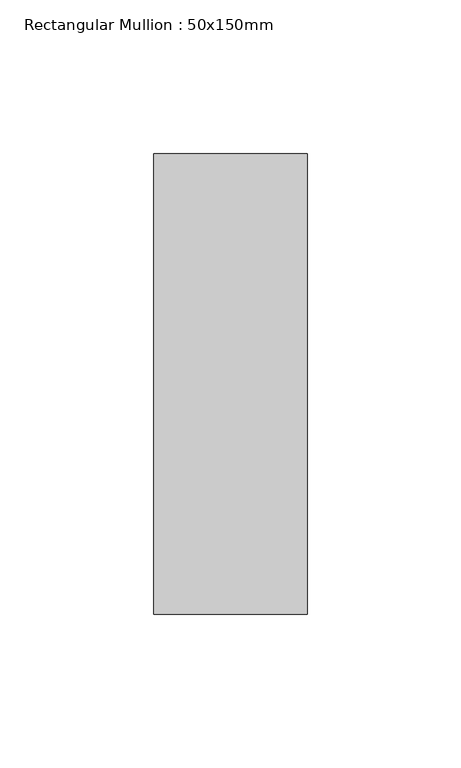
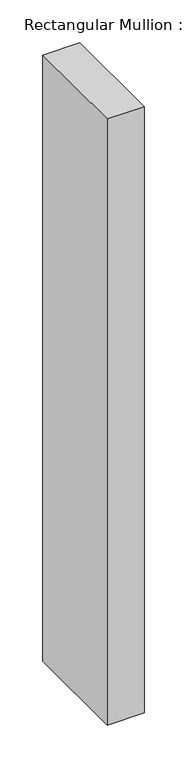
"""IFC4 building model written with IfcOpenShell, lengths in millimetres: member geometry, Rectangular Mullion : 50x150mm."""

from ifc_helpers import new_model, si_unit, frame, origin, place, context, project, spatial, polyline, outline, extrude, source, transform, mapped, element, save


def rectangular_mullion_50x150mm_5ffedf64(model_context):
    return source(origin(), model_context, "Body", "SweptSolid", [
        extrude(outline(polyline([(0.0, 75.0), (0.0, -75.0), (-50.0, -75.0), (-50.0, 75.0), (0.0, 75.0)])), frame((0.0, 0.0, -864.4), z_axis=(0.0, 0.0, 1.0), x_axis=(1.0, 0.0, 0.0)), (0.0, 0.0, 1.0), 864.4),
    ])


if __name__ == "__main__":
    model = new_model("IFC4")
    model_context = context("Model", 3, world=origin())
    ifc_project = project(units=[si_unit("LENGTHUNIT", "METRE", prefix="MILLI")], contexts=[model_context])
    site = spatial("IfcSite", under=ifc_project)
    building = spatial("IfcBuilding", under=site)
    placement = place(None, origin())
    rectangular_mullion_50x150mm_shape = rectangular_mullion_50x150mm_5ffedf64(model_context)
    element("IfcMember", 1, ObjectType="Rectangular Mullion : 50x150mm", at=placement, inside=building, context=model_context, shape_type="MappedRepresentation", body=[
        mapped(rectangular_mullion_50x150mm_shape, transform((0.0, 0.0, 0.0), x_axis=(1.0, 0.0, 0.0), y_axis=(0.0, 1.0, 0.0), z_axis=(0.0, 0.0, 1.0))),
    ])
    save(model, "model.ifc")

# Revit data of these elements
# Type "Rectangular Mullion : 50x150mm"
#   Keynote = "H11"
#   built-in parameter 1007304 = 0.492126 (stored number, unit not read)
#   built-in parameter 1007301 = 0.082021 (stored number, unit not read)
#   built-in parameter 1007300 = 0.082021 (stored number, unit not read)
# Element 1 (IfcMember, "Rectangular Mullion : 50x150mm")
#   Materials on its faces: "Aluminium"
# Materials
#   "Aluminium": class "Metal", colour RGB 247 247 247, transparency 0, Description = "Aluminium 6061", Cost = 0
